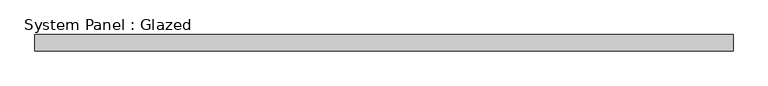
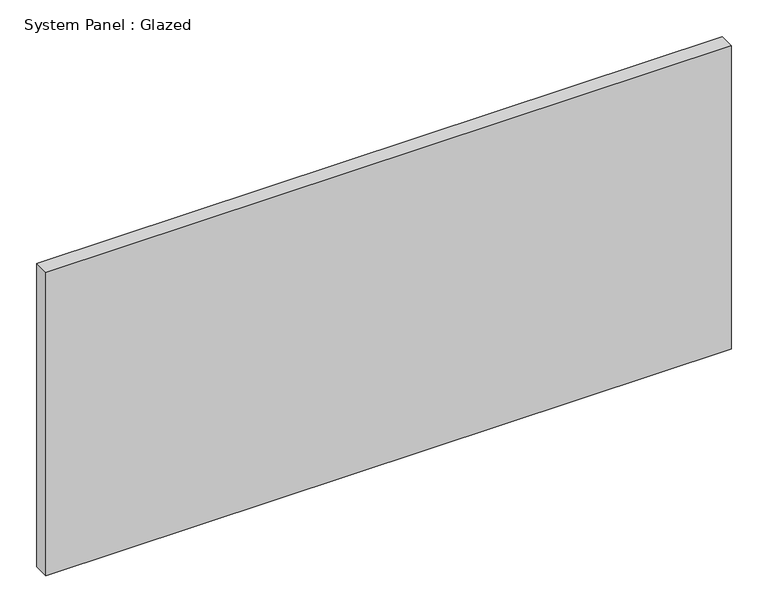
"""IFC4 building model written with IfcOpenShell, lengths in millimetres: plate geometry, System Panel : Glazed."""

from ifc_helpers import new_model, si_unit, origin, origin_with_axes, place, context, project, spatial, polyline, outline, extrude, source, transform, mapped, element, save


def system_panel_glazed_1a26cfa3(model_context):
    return source(origin(), model_context, "Body", "SweptSolid", [
        extrude(outline(polyline([(539.75, 19.05), (-539.75, 19.05), (-539.75, 44.45), (539.75, 44.45), (539.75, 19.05)])), origin_with_axes(), (0.0, 0.0, 1.0), 505.46),
    ])


if __name__ == "__main__":
    model = new_model("IFC4")
    model_context = context("Model", 3, world=origin())
    ifc_project = project(units=[si_unit("LENGTHUNIT", "METRE", prefix="MILLI")], contexts=[model_context])
    site = spatial("IfcSite", under=ifc_project)
    building = spatial("IfcBuilding", under=site)
    placement = place(None, origin())
    system_panel_glazed_shape = system_panel_glazed_1a26cfa3(model_context)
    element("IfcPlate", 1, ObjectType="System Panel : Glazed", at=placement, inside=building, context=model_context, shape_type="MappedRepresentation", body=[
        mapped(system_panel_glazed_shape, transform((0.0, 0.0, 0.0), x_axis=(1.0, 0.0, 0.0), y_axis=(0.0, 1.0, 0.0), z_axis=(0.0, 0.0, 1.0))),
    ])
    save(model, "model.ifc")

# Revit data of these elements
# Type "System Panel : Glazed"
#   Construction Type Id = "GSP4R"
#   Analytic Construction = "1/8 in Pilkington single glazing"
#   Visual Light Transmittance = 0.9
#   Solar Heat Gain Coefficient = 0.86
#   Heat Transfer Coefficient (U) = 1.18115 BTU/(h·ft²·°F)
#   Define Thermal Properties by = 1
# Element 1 (IfcPlate, "System Panel : Glazed")
#   Materials on its faces: "Glass"
# Materials
#   "Glass": class "Glass", colour RGB 0 128 192, transparency 0.75, Description = "Soda Lime Glass", Cost = 0
